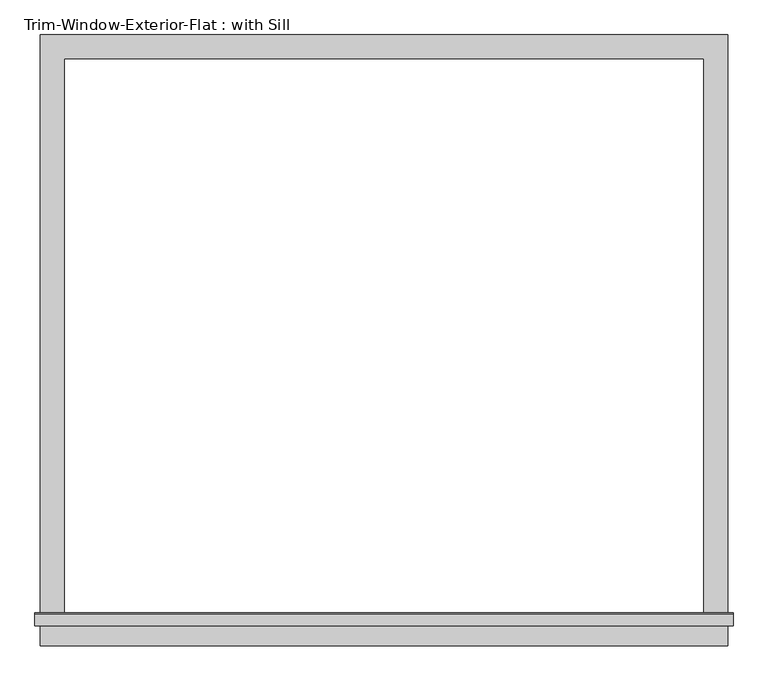
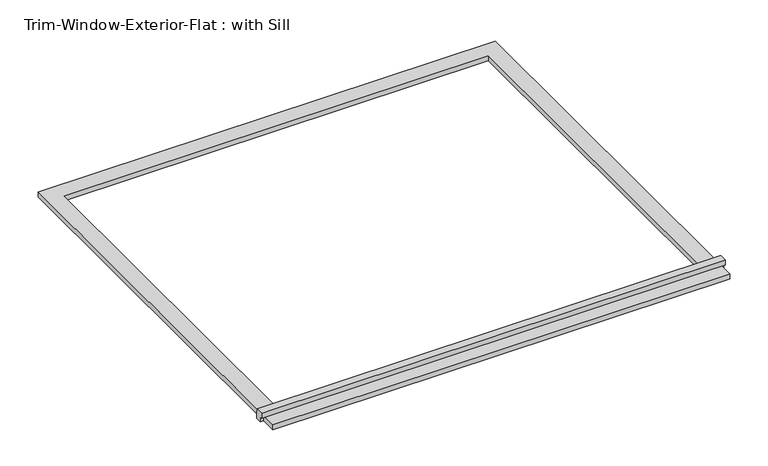
"""IFC4 building model written with IfcOpenShell, lengths in millimetres: proxy geometry, Trim-Window-Exterior-Flat : with Sill."""

from ifc_helpers import new_model, si_unit, frame, origin, origin_with_axes, place, context, project, spatial, polyline, outline, extrude, source, transform, mapped, element, save


def trim_window_exterior_flat_with_sill_5d4eb4de(model_context):
    return source(origin(), model_context, "Body", "SweptSolid", [
        extrude(outline(polyline([(819.15, -1342.9823709), (819.15, -1400.1323709), (-819.15, -1400.1323709), (-819.15, -1342.9823709), (819.15, -1342.9823709)])), origin_with_axes(), (0.0, 0.0, 1.0), 19.05),
        extrude(outline(polyline([(-1352.55, 38.1), (-1323.2580645, 38.1), (-1320.8, 19.05), (-1320.8, 0.0), (-1342.9823709, 0.0), (-1342.9823709, 19.05), (-1352.55, 19.05), (-1352.55, 38.1)])), frame((-831.85, 0.0, 0.0), z_axis=(1.0, 0.0, 0.0), x_axis=(0.0, 1.0, 0.0)), (0.0, 0.0, 1.0), 1663.7),
        extrude(outline(polyline([(-819.15, 57.15), (819.15, 57.15), (819.15, -1320.8), (762.0, -1320.8), (762.0, 0.0), (-762.0, 0.0), (-762.0, -1320.8), (-819.15, -1320.8), (-819.15, 57.15)])), origin_with_axes(), (0.0, 0.0, 1.0), 19.05),
    ])


if __name__ == "__main__":
    model = new_model("IFC4")
    model_context = context("Model", 3, world=origin())
    ifc_project = project(units=[si_unit("LENGTHUNIT", "METRE", prefix="MILLI")], contexts=[model_context])
    site = spatial("IfcSite", under=ifc_project)
    building = spatial("IfcBuilding", under=site)
    placement = place(None, origin())
    trim_window_exterior_flat_with_sill_shape = trim_window_exterior_flat_with_sill_5d4eb4de(model_context)
    element("IfcBuildingElementProxy", 1, Name="Trim-Window-Exterior-Flat : with Sill", ObjectType="Trim-Window-Exterior-Flat : with Sill", at=placement, inside=building, context=model_context, shape_type="MappedRepresentation", body=[
        mapped(trim_window_exterior_flat_with_sill_shape, transform((0.0, 0.0, 0.0), x_axis=(1.0, 0.0, 0.0), y_axis=(0.0, 1.0, 0.0), z_axis=(0.0, 0.0, 1.0))),
    ])
    save(model, "model.ifc")

# Revit data of these elements
# Type "Trim-Window-Exterior-Flat : with Sill"
#   Trim Width = 0' - 2 1/4"
#   Trim Thickness_Picture Frame = 0' - 1 1/4"
#   Trim Thickness_with Sill = 0' - 0 3/4"
#   Sill Thickness = 0' - 1 1/4"
#   Opening Width [instance default] = 2' - 0"
#   Opening Height [instance default] = 3' - 0"
#   Default Elevation = 4' - 0"
#   Sill = yes
#   Picture Frame = no
#   Trim Material [instance default] = none
# Element 1 (IfcBuildingElementProxy, "Trim-Window-Exterior-Flat : with Sill")
#   Opening Width = 5' - 0"
#   Opening Height = 4' - 4"
#   Trim Material = Clad - White
#   Materials on its faces: "Clad - White"
# Materials
#   "Clad - White": class "Wood", colour RGB 242 242 238, transparency 0, Cost = 0
